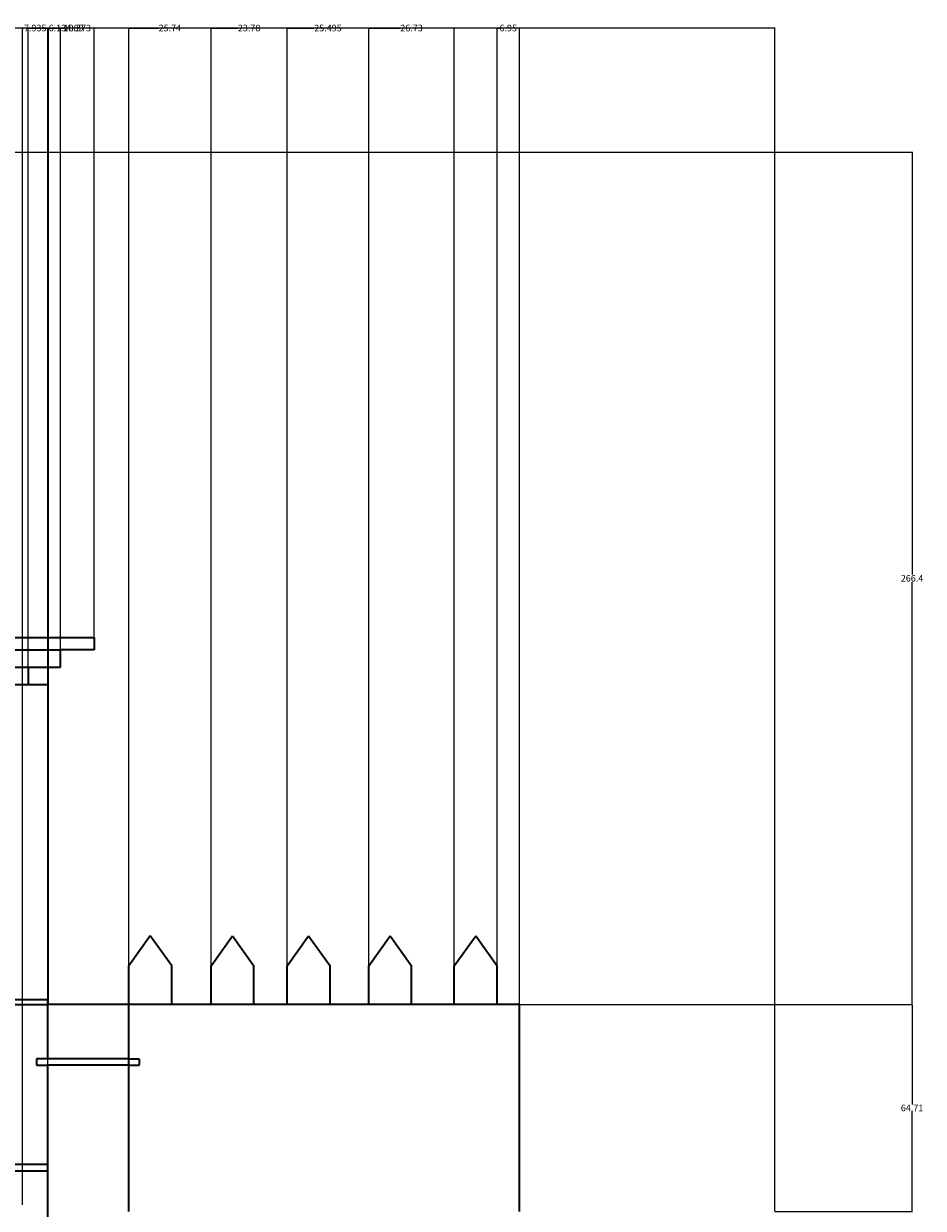
# Model space of a CAD drawing. Units: inches. Extents: x 14 to 859, y 52 to 711.
# Tile 11 of 11: x 577 to 858, y 341 to 711. Entities that reach past the tile are written whole.
import ezdxf

# ---------------------------------------------------------------- set-up
doc = ezdxf.new("R2010")
doc.units = ezdxf.units.IN
doc.header["$MEASUREMENT"] = 0
doc.layers.add('A-ANNO-DIMS', color=2, linetype='Continuous', lineweight=18)
doc.layers.add('A-ELEV', color=7, linetype='Continuous', lineweight=35)
doc.styles.get("Standard").update_dxf_attribs({"font": 'arial.ttf'})
doc.dimstyles.get("Standard").update_dxf_attribs({"dimtxt": 2.0625, "dimasz": 0.18, "dimexe": 0.18, "dimexo": 0.0625, "dimgap": 0.09, "dimtad": 0, "dimtih": 1, "dimtoh": 1, "dimdec": 4, "dimzin": 0, "dimdsep": 46, "dimlunit": 4, "dimtxsty": 'Standard', "dimcen": 0.09, "dimadec": 0, "dimazin": 0, "dimtfac": 1, "dimtdec": 4, "dimtofl": 0, "dimtmove": 0, "dimatfit": 3, "dimfxl": 1, "dimtolj": 1, "dimtzin": 0, "dimarcsym": 0})

# ---------------------------------------------------------------- blocks, each defined once
blk = doc.blocks.new('MERLON-SMALL')
for p, q in [((0, 12.05), (6.7, 21.41)), ((6.7, 21.41), (13.39, 12.05)), ((0, 0), (0, 12.05)), ((13.39, 0), (13.39, 12.05))]:
    blk.add_line(p, q)
blk = doc.blocks.new('*D13')
at = {"layer": 'A-ANNO-DIMS', "color": 0, "lineweight": -2, "transparency": 16777216}
for p, q in [((60.78, 339.73), (60.78, 709.71)), ((60.96, 709.53), (432.6, 709.53)), ((811.37, 709.53), (439.73, 709.53)), ((811.55, 339.73), (811.55, 709.71))]:
    blk.add_line(p, q, dxfattribs=at)
at = {"layer": 'A-ANNO-DIMS', "color": 0, "transparency": 16777216}
for points in [[(60.96, 709.56), (60.96, 709.5), (60.78, 709.53)], [(811.37, 709.56), (811.37, 709.5), (811.55, 709.53)]]:
    blk.add_solid(points, dxfattribs=at)
at = {"layer": 'Defpoints', "color": 0, "transparency": 16777216}
for p in [(811.55, 709.53), (60.78, 339.66), (811.55, 339.66)]:
    blk.add_point(p, dxfattribs=at)
at = {"layer": 'A-ANNO-DIMS', "color": 0, "transparency": 16777216, "insert": (436.17, 709.53), "char_height": 2.062, "attachment_point": 5}
blk.add_mtext('\\A1;750.8', dxfattribs=at)
blk = doc.blocks.new('*D18')
at = {"layer": 'A-ANNO-DIMS', "color": 0, "lineweight": -2, "transparency": 16777216}
for p, q in [((584.68, 404.37), (854.64, 404.37)), ((854.46, 404.19), (854.46, 373.16)), ((854.46, 339.84), (854.46, 370.87)), ((811.62, 339.66), (854.64, 339.66))]:
    blk.add_line(p, q, dxfattribs=at)
at = {"layer": 'A-ANNO-DIMS', "color": 0, "transparency": 16777216}
for points in [[(854.43, 404.19), (854.49, 404.19), (854.46, 404.37)], [(854.43, 339.84), (854.49, 339.84), (854.46, 339.66)]]:
    blk.add_solid(points, dxfattribs=at)
at = {"layer": 'Defpoints', "color": 0, "transparency": 16777216}
for p in [(584.62, 404.37), (854.46, 404.37), (811.55, 339.66)]:
    blk.add_point(p, dxfattribs=at)
at = {"layer": 'A-ANNO-DIMS', "color": 0, "transparency": 16777216, "insert": (854.46, 372.02), "char_height": 2.062, "attachment_point": 5}
blk.add_mtext('\\A1;64.71', dxfattribs=at)
blk = doc.blocks.new('*D19')
at = {"layer": 'A-ANNO-DIMS', "color": 0, "lineweight": -2, "transparency": 16777216}
for p, q in [((430.09, 670.76), (854.64, 670.76)), ((854.46, 670.58), (854.46, 538.71)), ((854.46, 404.55), (854.46, 536.42)), ((609.81, 404.37), (854.64, 404.37))]:
    blk.add_line(p, q, dxfattribs=at)
at = {"layer": 'A-ANNO-DIMS', "color": 0, "transparency": 16777216}
for points in [[(854.43, 670.58), (854.49, 670.58), (854.46, 670.76)], [(854.43, 404.55), (854.49, 404.55), (854.46, 404.37)]]:
    blk.add_solid(points, dxfattribs=at)
at = {"layer": 'Defpoints', "color": 0, "transparency": 16777216}
for p in [(430.02, 670.76), (854.46, 670.76), (609.75, 404.37)]:
    blk.add_point(p, dxfattribs=at)
at = {"layer": 'A-ANNO-DIMS', "color": 0, "transparency": 16777216, "insert": (854.46, 537.57), "char_height": 2.062, "attachment_point": 5}
blk.add_mtext('\\A1;266.4', dxfattribs=at)
blk = doc.blocks.new('*D23')
at = {"layer": 'A-ANNO-DIMS', "color": 0, "lineweight": -2, "transparency": 16777216}
for p, q in [((576.51, 341.73), (576.51, 709.71)), ((576.69, 709.53), (576.9, 709.53)), ((584.26, 709.53), (584.04, 709.53)), ((584.44, 352.49), (584.44, 709.71))]:
    blk.add_line(p, q, dxfattribs=at)
at = {"layer": 'A-ANNO-DIMS', "color": 0, "transparency": 16777216}
for points in [[(576.69, 709.56), (576.69, 709.5), (576.51, 709.53)], [(584.26, 709.56), (584.26, 709.5), (584.44, 709.53)]]:
    blk.add_solid(points, dxfattribs=at)
at = {"layer": 'Defpoints', "color": 0, "transparency": 16777216}
for p in [(584.44, 709.53), (584.44, 352.43), (576.51, 341.67)]:
    blk.add_point(p, dxfattribs=at)
at = {"layer": 'A-ANNO-DIMS', "color": 0, "transparency": 16777216, "insert": (580.47, 709.53), "char_height": 2.062, "attachment_point": 5}
blk.add_mtext('\\A1;7.935', dxfattribs=at)
blk = doc.blocks.new('*D80')
at = {"layer": 'A-ANNO-DIMS', "color": 0, "lineweight": -2, "transparency": 16777216}
for p, q in [((609.68, 404.43), (609.68, 709.71)), ((609.86, 709.53), (618.97, 709.53)), ((635.24, 709.53), (626.13, 709.53)), ((635.42, 404.43), (635.42, 709.71))]:
    blk.add_line(p, q, dxfattribs=at)
at = {"layer": 'A-ANNO-DIMS', "color": 0, "transparency": 16777216}
for points in [[(609.86, 709.56), (609.86, 709.5), (609.68, 709.53)], [(635.24, 709.56), (635.24, 709.5), (635.42, 709.53)]]:
    blk.add_solid(points, dxfattribs=at)
at = {"layer": 'Defpoints', "color": 0, "transparency": 16777216}
for p in [(635.42, 709.53), (609.68, 404.37), (635.42, 404.37)]:
    blk.add_point(p, dxfattribs=at)
at = {"layer": 'A-ANNO-DIMS', "color": 0, "transparency": 16777216, "insert": (622.55, 709.53), "char_height": 2.062, "attachment_point": 5}
blk.add_mtext('\\A1;25.74', dxfattribs=at)
blk = doc.blocks.new('*D81')
at = {"layer": 'A-ANNO-DIMS', "color": 0, "lineweight": -2, "transparency": 16777216}
for p, q in [((635.42, 404.43), (635.42, 709.71)), ((635.6, 709.53), (643.72, 709.53)), ((659.02, 709.53), (650.9, 709.53)), ((659.2, 404.43), (659.2, 709.71))]:
    blk.add_line(p, q, dxfattribs=at)
at = {"layer": 'A-ANNO-DIMS', "color": 0, "transparency": 16777216}
for points in [[(635.6, 709.56), (635.6, 709.5), (635.42, 709.53)], [(659.02, 709.56), (659.02, 709.5), (659.2, 709.53)]]:
    blk.add_solid(points, dxfattribs=at)
at = {"layer": 'Defpoints', "color": 0, "transparency": 16777216}
for p in [(659.2, 709.53), (635.42, 404.37), (659.2, 404.37)]:
    blk.add_point(p, dxfattribs=at)
at = {"layer": 'A-ANNO-DIMS', "color": 0, "transparency": 16777216, "insert": (647.31, 709.53), "char_height": 2.062, "attachment_point": 5}
blk.add_mtext('\\A1;23.78', dxfattribs=at)
blk = doc.blocks.new('*D82')
at = {"layer": 'A-ANNO-DIMS', "color": 0, "lineweight": -2, "transparency": 16777216}
for p, q in [((659.2, 404.43), (659.2, 709.71)), ((659.38, 709.53), (667.55, 709.53)), ((684.52, 709.53), (676.34, 709.53)), ((684.7, 404.43), (684.7, 709.71))]:
    blk.add_line(p, q, dxfattribs=at)
at = {"layer": 'A-ANNO-DIMS', "color": 0, "transparency": 16777216}
for points in [[(659.38, 709.56), (659.38, 709.5), (659.2, 709.53)], [(684.52, 709.56), (684.52, 709.5), (684.7, 709.53)]]:
    blk.add_solid(points, dxfattribs=at)
at = {"layer": 'Defpoints', "color": 0, "transparency": 16777216}
for p in [(684.7, 709.53), (659.2, 404.37), (684.7, 404.37)]:
    blk.add_point(p, dxfattribs=at)
at = {"layer": 'A-ANNO-DIMS', "color": 0, "transparency": 16777216, "insert": (671.95, 709.53), "char_height": 2.062, "attachment_point": 5}
blk.add_mtext('\\A1;25.495', dxfattribs=at)
blk = doc.blocks.new('*D83')
at = {"layer": 'A-ANNO-DIMS', "color": 0, "lineweight": -2, "transparency": 16777216}
for p, q in [((684.7, 404.43), (684.7, 709.71)), ((684.88, 709.53), (694.47, 709.53)), ((711.25, 709.53), (701.65, 709.53)), ((711.43, 404.43), (711.43, 709.71))]:
    blk.add_line(p, q, dxfattribs=at)
at = {"layer": 'A-ANNO-DIMS', "color": 0, "transparency": 16777216}
for points in [[(684.88, 709.56), (684.88, 709.5), (684.7, 709.53)], [(711.25, 709.56), (711.25, 709.5), (711.43, 709.53)]]:
    blk.add_solid(points, dxfattribs=at)
at = {"layer": 'Defpoints', "color": 0, "transparency": 16777216}
for p in [(711.43, 709.53), (684.7, 404.37), (711.43, 404.37)]:
    blk.add_point(p, dxfattribs=at)
at = {"layer": 'A-ANNO-DIMS', "color": 0, "transparency": 16777216, "insert": (698.06, 709.53), "char_height": 2.062, "attachment_point": 5}
blk.add_mtext('\\A1;26.73', dxfattribs=at)
blk = doc.blocks.new('*D84')
at = {"layer": 'A-ANNO-DIMS', "color": 0, "lineweight": -2, "transparency": 16777216}
for p, q in [((724.82, 404.43), (724.82, 709.71)), ((725, 709.53), (725.51, 709.53)), ((731.59, 709.53), (731.07, 709.53)), ((731.77, 404.43), (731.77, 709.71))]:
    blk.add_line(p, q, dxfattribs=at)
at = {"layer": 'A-ANNO-DIMS', "color": 0, "transparency": 16777216}
for points in [[(725, 709.56), (725, 709.5), (724.82, 709.53)], [(731.59, 709.56), (731.59, 709.5), (731.77, 709.53)]]:
    blk.add_solid(points, dxfattribs=at)
at = {"layer": 'Defpoints', "color": 0, "transparency": 16777216}
for p in [(731.77, 709.53), (724.82, 404.37), (731.77, 404.37)]:
    blk.add_point(p, dxfattribs=at)
at = {"layer": 'A-ANNO-DIMS', "color": 0, "transparency": 16777216, "insert": (728.29, 709.53), "char_height": 2.062, "attachment_point": 5}
blk.add_mtext('\\A1;6.95', dxfattribs=at)
blk = doc.blocks.new('*D100')
at = {"layer": 'A-ANNO-DIMS', "color": 0, "lineweight": -2, "transparency": 16777216}
for p, q in [((547.09, 509.85), (547.09, 709.71)), ((547.27, 709.53), (561.39, 709.53)), ((584.26, 709.53), (570.13, 709.53)), ((584.44, 504.44), (584.44, 709.71))]:
    blk.add_line(p, q, dxfattribs=at)
at = {"layer": 'A-ANNO-DIMS', "color": 0, "transparency": 16777216}
for points in [[(547.27, 709.56), (547.27, 709.5), (547.09, 709.53)], [(584.26, 709.56), (584.26, 709.5), (584.44, 709.53)]]:
    blk.add_solid(points, dxfattribs=at)
at = {"layer": 'Defpoints', "color": 0, "transparency": 16777216}
for p in [(584.44, 709.53), (547.09, 509.79), (584.44, 504.38)]:
    blk.add_point(p, dxfattribs=at)
at = {"layer": 'A-ANNO-DIMS', "color": 0, "transparency": 16777216, "insert": (565.76, 709.53), "char_height": 2.062, "attachment_point": 5}
blk.add_mtext('\\A1;37.356', dxfattribs=at)
blk = doc.blocks.new('*D101')
at = {"layer": 'A-ANNO-DIMS', "color": 0, "lineweight": -2, "transparency": 16777216}
for p, q in [((578.31, 509.85), (578.31, 709.71)), ((578.49, 709.53), (584.26, 709.53)), ((584.44, 504.44), (584.44, 709.71)), ((584.44, 709.53), (584.62, 709.53))]:
    blk.add_line(p, q, dxfattribs=at)
at = {"layer": 'A-ANNO-DIMS', "color": 0, "transparency": 16777216}
for points in [[(578.49, 709.56), (578.49, 709.5), (578.31, 709.53)], [(584.26, 709.56), (584.26, 709.5), (584.44, 709.53)]]:
    blk.add_solid(points, dxfattribs=at)
at = {"layer": 'Defpoints', "color": 0, "transparency": 16777216}
for p in [(584.44, 709.53), (578.31, 509.79), (584.44, 504.38)]:
    blk.add_point(p, dxfattribs=at)
at = {"layer": 'A-ANNO-DIMS', "color": 0, "transparency": 16777216, "insert": (588.19, 709.53), "char_height": 2.062, "attachment_point": 5}
blk.add_mtext('\\A1;6.134', dxfattribs=at)
blk = doc.blocks.new('*D102')
at = {"layer": 'A-ANNO-DIMS', "color": 0, "lineweight": -2, "transparency": 16777216}
for p, q in [((584.44, 504.44), (584.44, 709.71)), ((584.62, 709.53), (588.15, 709.53)), ((588.33, 515.26), (588.33, 709.71)), ((588.33, 709.53), (588.51, 709.53))]:
    blk.add_line(p, q, dxfattribs=at)
at = {"layer": 'A-ANNO-DIMS', "color": 0, "transparency": 16777216}
for points in [[(584.62, 709.56), (584.62, 709.5), (584.44, 709.53)], [(588.15, 709.56), (588.15, 709.5), (588.33, 709.53)]]:
    blk.add_solid(points, dxfattribs=at)
at = {"layer": 'Defpoints', "color": 0, "transparency": 16777216}
for p in [(588.33, 709.53), (588.33, 515.2), (584.44, 504.38)]:
    blk.add_point(p, dxfattribs=at)
at = {"layer": 'A-ANNO-DIMS', "color": 0, "transparency": 16777216, "insert": (592.08, 709.53), "char_height": 2.062, "attachment_point": 5}
blk.add_mtext('\\A1;3.889', dxfattribs=at)
blk = doc.blocks.new('*D103')
at = {"layer": 'A-ANNO-DIMS', "color": 0, "lineweight": -2, "transparency": 16777216}
for p, q in [((588.33, 515.26), (588.33, 709.71)), ((588.51, 709.53), (589.34, 709.53)), ((598.72, 709.53), (597.89, 709.53)), ((598.9, 519.11), (598.9, 709.71))]:
    blk.add_line(p, q, dxfattribs=at)
at = {"layer": 'A-ANNO-DIMS', "color": 0, "transparency": 16777216}
for points in [[(588.51, 709.56), (588.51, 709.5), (588.33, 709.53)], [(598.72, 709.56), (598.72, 709.5), (598.9, 709.53)]]:
    blk.add_solid(points, dxfattribs=at)
at = {"layer": 'Defpoints', "color": 0, "transparency": 16777216}
for p in [(598.9, 709.53), (598.9, 519.05), (588.33, 515.2)]:
    blk.add_point(p, dxfattribs=at)
at = {"layer": 'A-ANNO-DIMS', "color": 0, "transparency": 16777216, "insert": (593.62, 709.53), "char_height": 2.062, "attachment_point": 5}
blk.add_mtext('\\A1;10.573', dxfattribs=at)
blk = doc.blocks.new('*D123')
at = {"layer": 'A-ANNO-DIMS', "color": 0, "lineweight": -2, "transparency": 16777216}
for p, q in [((539.45, 404.43), (539.45, 709.71)), ((539.63, 709.53), (558.42, 709.53)), ((584.44, 709.53), (565.64, 709.53)), ((584.62, 404.43), (584.62, 709.71))]:
    blk.add_line(p, q, dxfattribs=at)
at = {"layer": 'A-ANNO-DIMS', "color": 0, "transparency": 16777216}
for points in [[(539.63, 709.56), (539.63, 709.5), (539.45, 709.53)], [(584.44, 709.56), (584.44, 709.5), (584.62, 709.53)]]:
    blk.add_solid(points, dxfattribs=at)
at = {"layer": 'Defpoints', "color": 0, "transparency": 16777216}
for p in [(584.62, 709.53), (539.45, 404.37), (584.62, 404.37)]:
    blk.add_point(p, dxfattribs=at)
at = {"layer": 'A-ANNO-DIMS', "color": 0, "transparency": 16777216, "insert": (562.03, 709.53), "char_height": 2.062, "attachment_point": 5}
blk.add_mtext('\\A1;45.17', dxfattribs=at)

msp = doc.modelspace()

# ---------------------------------------------------------------- linework, layer by layer
at = {"layer": 'A-ELEV'}
for p, q in [((555.2103, 519.0512), (598.9032, 519.0512)), ((598.9032, 519.0512), (598.9032, 515.1991)), ((537.6873, 515.1991), (588.3297, 515.1991)), ((588.3297, 515.1991), (588.3297, 515.1991)), ((588.3297, 509.7903), (588.3297, 515.1991)), ((598.9032, 515.1991), (588.3297, 515.1991)), ((537.6873, 509.7903), (578.3064, 509.7903)), ((578.3064, 509.7903), (578.3064, 504.3815)), ((578.3064, 509.7903), (588.3297, 509.7903)), ((536.2033, 504.3815), (584.4409, 504.3815)), ((584.4409, 504.3815), (584.4409, 405.9412)), ((616.445, 425.7853), (609.7501, 416.4248)), ((623.1399, 416.4248), (616.445, 425.7853)), ((609.7501, 404.3712), (609.7501, 416.4248)), ((623.1399, 404.3712), (623.1399, 416.4248)), ((376.0525, 404.3712), (584.619, 404.3712)), ((539.446, 405.9412), (584.4409, 405.9412)), ((584.4409, 387.3985), (584.4409, 405.9412)), ((609.6802, 404.3712), (584.4409, 404.3712)), ((609.6802, 370.2389), (609.6802, 404.3712)), ((731.7655, 404.3712), (609.6802, 404.3712)), ((731.7655, 339.6626), (731.7655, 404.3712)), ((584.4409, 387.3985), (580.8768, 387.3985)), ((580.8768, 387.3985), (580.8768, 385.3985)), ((580.8768, 385.3985), (584.4409, 385.3985)), ((609.6802, 387.3985), (584.4409, 387.3985)), ((584.4409, 371.6812), (584.4409, 385.3985)), ((609.6802, 385.3985), (584.4409, 385.3985)), ((609.6802, 387.3985), (612.912, 387.3985)), ((609.6802, 385.3985), (612.912, 385.3985)), ((612.912, 387.3985), (612.912, 385.3985)), ((584.4409, 304.6217), (584.4409, 371.6812)), ((609.6802, 339.6626), (609.6802, 370.2389)), ((287.893, 354.4291), (584.4409, 354.4291)), ((287.893, 352.4291), (584.4409, 352.4291))]:
    msp.add_line(p, q, dxfattribs=at)

# ---------------------------------------------------------------- block references
for p in [(635.4181, 404.371), (659.1999, 404.371), (684.6949, 404.371), (711.4255, 404.371)]:
    msp.add_blockref('MERLON-SMALL', p, dxfattribs=at)

# ---------------------------------------------------------------- dimensions: what is measured, and where the dimension line sits
at = {"layer": 'A-ANNO-DIMS'}
for base, p1, p2, override, picture, middle in [((811.5534, 709.5262), (60.7804, 339.6626), (811.5534, 339.6626), {"dimdec": 1, "dimlfac": 1, "dimrnd": 0, "dimzin": 0, "dimdsep": 46, "dimlunit": 2}, '*D13', (436.1669, 709.5262)), ((584.619, 709.5262), (539.446, 404.3712), (584.619, 404.3712), {"dimdec": 2, "dimlfac": 1, "dimrnd": 0, "dimzin": 0, "dimdsep": 46, "dimlunit": 2}, '*D123', (562.0325, 709.5262)), ((584.4409, 709.5262), (547.0851, 509.7903), (584.4409, 504.3815), {"dimdec": 3, "dimlfac": 1, "dimrnd": 0, "dimzin": 0, "dimdsep": 46, "dimlunit": 2}, '*D100', (565.763, 709.5262)), ((584.4409, 709.5262), (576.5058, 341.6716), (584.4409, 352.4291), {"dimdec": 3, "dimlfac": 1, "dimrnd": 0, "dimzin": 0, "dimdsep": 46, "dimlunit": 2}, '*D23', (580.4733, 709.5262)), ((584.44087, 709.52622), (578.30642, 509.79029), (584.44087, 504.38152), {"dimdec": 3, "dimlfac": 1, "dimrnd": 0, "dimzin": 0, "dimdsep": 46, "dimlunit": 2}, '*D101', (588.19222, 709.52622)), ((588.3297, 709.5262), (584.4409, 504.3815), (588.3297, 515.1991), {"dimdec": 3, "dimlfac": 1, "dimrnd": 0, "dimzin": 0, "dimdsep": 46, "dimlunit": 2}, '*D102', (592.0811, 709.5262)), ((598.9032, 709.52622), (588.32971, 515.19905), (598.9032, 519.05118), {"dimdec": 3, "dimlfac": 1, "dimrnd": 0, "dimzin": 0, "dimdsep": 46, "dimlunit": 2}, '*D103', (593.61646, 709.52622)), ((635.4184, 709.5262), (609.6802, 404.3712), (635.4184, 404.3712), {"dimdec": 2, "dimlfac": 1, "dimrnd": 0, "dimzin": 0, "dimdsep": 46, "dimlunit": 2}, '*D80', (622.5493, 709.5262)), ((659.2001, 709.5262), (635.4184, 404.3712), (659.2001, 404.3712), {"dimdec": 2, "dimlfac": 1, "dimrnd": 0, "dimzin": 0, "dimdsep": 46, "dimlunit": 2}, '*D81', (647.3093, 709.5262)), ((684.6952, 709.5262), (659.2001, 404.3712), (684.6952, 404.3712), {"dimdec": 3, "dimlfac": 1, "dimrnd": 0, "dimzin": 0, "dimdsep": 46, "dimlunit": 2}, '*D82', (671.9477, 709.5262)), ((711.4257, 709.5262), (684.6952, 404.3712), (711.4257, 404.3712), {"dimdec": 2, "dimlfac": 1, "dimrnd": 0, "dimzin": 0, "dimdsep": 46, "dimlunit": 2}, '*D83', (698.0605, 709.5262)), ((731.7655, 709.5262), (724.8156, 404.3712), (731.7655, 404.3712), {"dimdec": 2, "dimlfac": 1, "dimrnd": 0, "dimzin": 0, "dimdsep": 46, "dimlunit": 2}, '*D84', (728.2906, 709.5262))]:
    dim = msp.add_linear_dim(base=base, p1=p1, p2=p2, dimstyle='Standard', override=override, dxfattribs=at)
    dim.commit()
    dim.dimension.update_dxf_attribs({"geometry": picture, "text_midpoint": middle})
for base, p1, p2, override, picture, middle in [((854.4554, 670.7637), (609.7501, 404.3712), (430.0228, 670.7637), {"dimdec": 1, "dimlfac": 1, "dimrnd": 0, "dimzin": 0, "dimdsep": 46, "dimlunit": 2}, '*D19', (854.4554, 537.5675)), ((854.4554, 404.3712), (811.5534, 339.6626), (584.619, 404.3712), {"dimdec": 2, "dimlfac": 1, "dimrnd": 0, "dimzin": 0, "dimdsep": 46, "dimlunit": 2}, '*D18', (854.4554, 372.0169))]:
    dim = msp.add_linear_dim(base=base, p1=p1, p2=p2, angle=90, dimstyle='Standard', override=override, dxfattribs=at)
    dim.commit()
    dim.dimension.update_dxf_attribs({"geometry": picture, "text_midpoint": middle})

doc.saveas('drawing.dxf')
